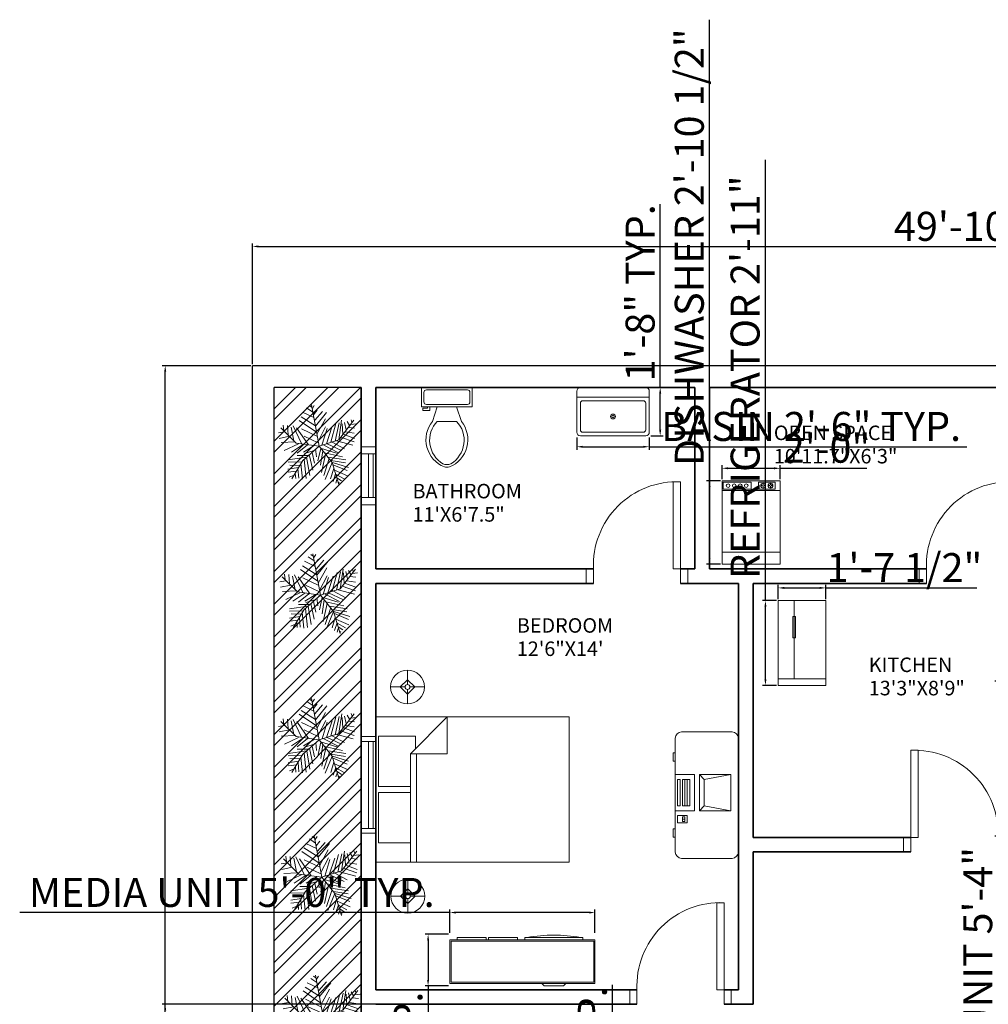
# Model space of a CAD drawing. Units: inches. Extents: x 2297 to 3143, y 440 to 1351.
# Tile 5 of 6: x 2297 to 2697, y 944 to 1351. Entities that reach past the tile are written whole.
import ezdxf

# ---------------------------------------------------------------- set-up
doc = ezdxf.new("R2010")
doc.units = ezdxf.units.IN
for name, color, linetype, lineweight in [('A-ANNO-DIMS', 2, 'Continuous', 18), ('A-AREA-IDEN', 7, 'Continuous', 18), ('A-DOOR', 4, 'Continuous', 20), ('A-EQPM', 8, 'Continuous', 18), ('A-FLOR-FIXT', 9, 'Continuous', 18), ('A-FURN', 8, 'Continuous', 18), ('A-GLAZ', 4, 'Continuous', 18), ('A-WALL', 7, 'Continuous', 35), ('C-PROP', 7, 'Continuous', 25), ('C-SITE-PATT', 252, 'Continuous', 13), ('E-LITE', 9, 'Continuous', 13), ('L-PLNT', 3, 'Continuous', 13)]:
    doc.layers.add(name, color=color, linetype=linetype, lineweight=lineweight)
doc.styles.get("Standard").update_dxf_attribs({"font": 'arial.ttf'})
doc.dimstyles.new('ISO-25', dxfattribs={"dimtxt": 12, "dimasz": 2.5, "dimexe": 1.25, "dimexo": 0.625, "dimtad": 1, "dimdec": 1, "dimlunit": 3, "dimtxsty": 'Standard', "dimcen": 2.5, "dimadec": 0, "dimazin": 0, "dimtfac": 1, "dimtdec": 1, "dimtmove": 0, "dimatfit": 3, "dimfxl": 1, "dimarcsym": 0})

# ---------------------------------------------------------------- blocks, each defined once
blk = doc.blocks.new('Bed - Queen')
for p, q in [((0, -80.00003), (0, 0)), ((0, 0), (59.99999, 0)), ((59.99999, 0), (59.99999, -80.00003)), ((7.99999, -1.2), (28.79998, -1.2)), ((7.99999, -14.4), (7.99999, -1.2)), ((28.79998, -1.2), (28.79998, -14.4)), ((31.19999, -1.2), (51.99999, -1.2)), ((31.19999, -14.4), (31.19999, -1.2)), ((51.99999, -1.2), (51.99999, -16.4)), ((0, -14.4), (44.8, -14.4)), ((59.99999, -29.6), (44.8, -14.4)), ((44.8, -14.4), (44.8, -29.6)), ((44.8, -16.8), (0, -16.8)), ((51.99999, -16.4), (46.79936, -16.4)), ((44.8, -29.6), (59.99999, -29.6)), ((59.99999, -80.00003), (0, -80.00003))]:
    blk.add_line(p, q)
blk = doc.blocks.new('Sink-single - 30 in top')
blk.add_line((-15, -3.999996), (15, -3.999996))
for points in [[(-13.5, 0), (13.5, 0)], [(-15, -18.499996), (-15, -1.5)], [(15, -1.5), (15, -18.499996)], [(-13.5, -17.499996), (-13.5, -6.499996)], [(-12.5, -5.499996), (12.5, -5.499996)], [(13.5, -6.499996), (13.5, -17.499996)], [(13.5, -19.999996), (-13.5, -19.999996)], [(12.5, -18.499996), (-12.5, -18.499996)]]:
    blk.add_lwpolyline(points)
for radius in [1, 0.5]:
    blk.add_circle((0, -11.999996), radius)
for centre, radius, start, end in [((-13.5, -1.5), 1.5, 90, 180), ((13.5, -1.5), 1.5, 0, 90), ((-12.5, -6.499996), 1, 90, 180), ((12.5, -6.499996), 1, 0, 90), ((-13.5, -18.499996), 1.5, 180, 270), ((-12.5, -17.499996), 1, 180, 270), ((12.5, -17.499996), 1, 270, 0), ((13.5, -18.499996), 1.5, 270, 0)]:
    blk.add_arc(centre, radius, start, end)
blk = doc.blocks.new('Toilet - top')
for p, q in [((9.5, -6), (9.5, -2)), ((-8, -8.5), (-8, -8)), ((-7, -8), (-7, -9.5)), ((-4, -8), (-6, -14)), ((4, -8), (6, -14)), ((-10, -8.5), (-8, -8.5)), ((-10, -9.5), (-10, -8.5)), ((-7, -9.5), (-10, -9.5)), ((4, -14), (-4, -14))]:
    blk.add_line(p, q)
blk.add_lwpolyline([(10.5, -8), (10.5, 0), (-10.5, 0), (-10.5, -8)], close=True)
for points in [[(-9.5, -2), (-9.5, -6)], [(8.5, -1), (-8.5, -1)], [(-8.5, -7), (8.5, -7)]]:
    blk.add_lwpolyline(points)
for centre, radius, start, end in [((-8.62, -1.88), 0.884, 81.8699, 188.1301), ((8.62, -1.88), 0.884, 351.8699, 98.1301), ((-8.62, -6.12), 0.884, 171.8699, 278.1301), ((8.62, -6.12), 0.884, 261.8699, 8.1301), ((3.52, -21.58), 12.17, 141.4691, 247.9714), ((4.2, -21.82), 11.33, 136.3677, 238.9468), ((-3.52, -21.58), 12.17, 292.0284, 38.5307), ((-4.2, -21.82), 11.33, 301.053, 43.6321), ((0, -27.88), 4, 245.7318, 294.2682), ((0, -29), 4, 254.8605, 285.1395)]:
    blk.add_arc(centre, radius, start, end)
blk = doc.blocks.new('*U16')
for p, q in [((-10.186, 53.64), (-13.084, 55.962)), ((0, 0), (-10.5, 57)), ((-9.099, 51.782), (-6.563, 55.962)), ((-7.288, 39.707), (-21.778, 46.673)), ((-8.737, 47.138), (-17.069, 52.711)), ((-7.65, 43.423), (-2.578, 49.46)), ((-5.839, 35.992), (4.667, 48.067)), ((-5.114, 27.632), (10.463, 46.673)), ((-48.585, 21.131), (-49.309, 29.026)), ((-43.513, 28.561), (-42.427, 15.558)), ((-35.544, 28.097), (-24.314, 3.947)), ((-3.665, 19.273), (-27.574, 35.527)), ((-5.114, 28.097), (-24.676, 40.636)), ((-2.941, 16.486), (8.652, 37.85)), ((16.259, 5.805), (23.142, 31.348)), ((22.055, 7.198), (27.489, 32.277)), ((27, 9), (48, 36)), ((27.127, 9.056), (31.112, 35.992)), ((31.836, 30.883), (32.561, 16.486)), ((35.096, 32.741), (37.27, 22.524)), ((38.719, 34.134), (41.979, 28.561)), ((43.791, 29.954), (51.036, 30.883)), ((44.153, 36.456), (45.239, 32.741)), ((-47.498, 19.737), (-55.83, 18.344)), ((-40.615, 13.7), (-55.105, 10.913)), ((-31.5, 4.5), (-52.5, 25.5)), ((-38.442, 26.239), (-34.819, 7.663)), ((-14.533, 2.09), (-30.834, 25.31)), ((-24.314, 23.917), (-2.941, 13.7)), ((-20.691, 13.7), (-1.129, 4.876)), ((-1.129, 6.734), (9.014, 26.704)), ((3.942, 1.625), (11.187, 24.381)), ((10.101, 3.483), (17.708, 26.239)), ((33.285, 16.486), (48.862, 10.913)), ((36.183, 19.737), (48.137, 17.88)), ((40.53, 25.775), (48.862, 24.846)), ((-33.37, 6.269), (-52.207, 5.34)), ((-28.299, 3.483), (-47.86, -5.805)), ((-21.416, 3.018), (-38.079, -8.128)), ((0, 0), (-31.5, 4.5)), ((-15.982, 2.09), (-30.11, -9.521)), ((0, 0), (-22.5, -19.5)), ((-6.563, 1.161), (-21.416, -8.128)), ((0, 0), (27, 9)), ((0, 0), (18, -22.5)), ((6.478, 1.625), (26.04, -8.592)), ((11.187, 3.483), (30.749, -5.805)), ((18.07, 5.805), (35.096, -3.483)), ((24.229, 7.663), (46.688, 1.625)), ((29.662, 12.307), (48.137, 6.269)), ((-15.257, -12.772), (-30.11, -12.772)), ((-6.563, -5.805), (-19.967, -9.985)), ((-13.446, -11.378), (-8.737, -32.741)), ((-9.461, -8.592), (-6.201, -23.453)), ((-4.752, -3.483), (-3.665, -14.629)), ((2.493, -3.019), (-1.491, -20.202)), ((1.769, -2.555), (24.229, -9.521)), ((5.029, -6.27), (2.131, -25.775)), ((9.014, -11.378), (3.58, -35.992)), ((7.565, -9.056), (32.198, -14.629)), ((-17.431, -15.094), (-42.789, -18.809)), ((-24.314, -21.596), (-42.427, -22.06)), ((-26.849, -26.24), (-40.253, -25.775)), ((-22.5, -19.5), (-37.5, -45)), ((-25.038, -23.918), (-22.865, -45.281)), ((-20.691, -18.345), (-17.793, -44.352)), ((-17.069, -15.094), (-12.721, -40.172)), ((14.085, -16.951), (6.478, -40.172)), ((18.07, -22.524), (8.289, -45.745)), ((12.274, -15.094), (36.907, -18.809)), ((16.259, -19.738), (36.183, -22.989)), ((18, -22.5), (27, -52.5)), ((18.433, -22.524), (40.53, -29.026)), ((19.157, -25.311), (38.719, -33.206)), ((-28.299, -29.026), (-42.789, -31.348)), ((-30.834, -34.135), (-42.427, -35.528)), ((-34.457, -39.708), (-40.978, -42.494)), ((-32.646, -36.921), (-31.921, -44.352)), ((-29.023, -30.884), (-27.936, -43.887)), ((20.244, -30.419), (15.897, -44.816)), ((22.78, -37.85), (19.519, -48.532)), ((21.331, -32.741), (39.081, -40.636)), ((22.78, -38.314), (34.372, -44.816)), ((24.591, -45.745), (23.142, -50.854)), ((24.591, -43.423), (30.749, -47.603)), ((26.764, -49.925), (28.213, -50.854))]:
    blk.add_line(p, q)
blk = doc.blocks.new('*D17')
at = {"layer": 'A-ANNO-DIMS', "color": 0, "lineweight": -2, "transparency": 16777216}
for p, q in [((2393.19, 1208.26), (2393.19, 1258.2)), ((2991.69, 1208.26), (2991.69, 1258.2)), ((2395.69, 1256.95), (2989.19, 1256.95))]:
    blk.add_line(p, q, dxfattribs=at)
at = {"layer": 'A-ANNO-DIMS', "color": 0, "transparency": 16777216}
for points in [[(2395.69, 1257.36), (2395.69, 1256.53), (2393.19, 1256.95)], [(2989.19, 1257.36), (2989.19, 1256.53), (2991.69, 1256.95)]]:
    blk.add_solid(points, dxfattribs=at)
at = {"layer": 'Defpoints', "color": 0, "transparency": 16777216}
for p in [(2991.69, 1256.95), (2393.19, 1207.63), (2991.69, 1207.63)]:
    blk.add_point(p, dxfattribs=at)
at = {"layer": 'A-ANNO-DIMS', "color": 0, "transparency": 16777216, "insert": (2692.44, 1263.7), "char_height": 12, "attachment_point": 5}
blk.add_mtext('49\'-10.5"', dxfattribs=at)
blk = doc.blocks.new('Lamp - Table')
for p, q in [((0, 7), (0, 1)), ((-1, 0), (-7, 0)), ((0, 3), (-3, 0)), ((-3, 0), (0, -3)), ((3, 0), (0, 3)), ((0, -3), (3, 0)), ((1, 0), (7, 0)), ((0, -1), (0, -7))]:
    blk.add_line(p, q)
for radius in [7, 1]:
    blk.add_circle((0, 0), radius)
blk = doc.blocks.new('Refrigerator-2 door - 36 in front')
for p, q in [((12, 5), (12, 64)), ((0, 5), (36, 5))]:
    blk.add_line(p, q)
for points in [[(0, 0), (0, 64), (36, 64), (36, 0)], [(11, 36), (11, 52), (13, 52), (13, 36)]]:
    blk.add_lwpolyline(points, close=True)
blk = doc.blocks.new('Desk - 30 x 60 in.')
for p, q in [((-26.999995, 0), (26.999995, 0)), ((-29.999995, -27), (-29.999995, -3)), ((29.999995, -3), (29.999995, -27)), ((26.999995, -30), (-26.999995, -30)), ((-20.000005, -30), (-20.000005, -31)), ((-20.000005, -31), (-16.000005, -31)), ((-16.000005, -31), (-16.000005, -30)), ((15.999995, -31), (15.999995, -30)), ((19.999995, -31), (15.999995, -31)), ((19.999995, -30), (19.999995, -31))]:
    blk.add_line(p, q)
for centre, start, end in [((-26.499995, -3.5), 98.1301, 171.8699), ((26.499995, -3.5), 8.130102, 81.8699), ((-26.499995, -26.5), 188.1301, 261.8699), ((26.499995, -26.5), 278.1301, 351.8699)]:
    blk.add_arc(centre, 3.535534, start, end)
blk = doc.blocks.new('Computer Terminal')
for p, q in [((-10, 11.5), (5, 11.5)), ((-8, 0.5), (-10, 11.5)), ((-10, -1.5), (-10, 11.5)), ((5, 11.5), (3, 0.5)), ((5, 11.5), (5, -1.5)), ((-10, -1.5), (-8, 0.5)), ((3, 0.5), (-8, 0.5)), ((3, 0.5), (5, -1.5)), ((5, -1.5), (-10, -1.5)), ((-10, -11.5), (-10, -3.5)), ((-10, -3.5), (5, -3.5)), ((5, -3.5), (5, -11.5)), ((-8, -5.5), (-8, -8.5)), ((3, -5.5), (-8, -5.5)), ((3, -6.5), (-8, -6.5)), ((-8, -7.5), (3, -7.5)), ((3, -8.5), (3, -5.5)), ((10, -6.5), (7, -6.5)), ((7, -6.5), (7, -10.5)), ((9.5, -7.5), (7.5, -7.5)), ((7.5, -7.5), (7.5, -8.5)), ((8.5, -7.5), (8.5, -8.5)), ((9.5, -8.5), (9.5, -7.5)), ((10, -10.5), (10, -6.5)), ((5, -11.5), (-10, -11.5)), ((-8, -8.5), (3, -8.5)), ((-8, -9.5), (-8, -10.5)), ((3, -9.5), (-8, -9.5)), ((-8, -10.5), (3, -10.5)), ((3, -10.5), (3, -9.5)), ((7, -10.5), (10, -10.5)), ((7.5, -8.5), (9.5, -8.5))]:
    blk.add_line(p, q)
blk = doc.blocks.new('Dishwasher')
for p, q in [((16.3156, 33.1843), (16.5, 33)), ((17, 32.75), (17, 33.5)), ((17.5, 33), (17.6938, 33.1938)), ((19.3156, 33.1843), (19.5, 33)), ((20, 32.75), (20, 33.5)), ((20.5, 33), (20.6938, 33.1938)), ((24, 30.5), (0, 30.5)), ((16, 32.5), (16.75, 32.5)), ((16.5, 32), (16.2942, 31.7942)), ((17, 32.25), (17, 31.5)), ((18, 32.5), (17.25, 32.5)), ((17.7061, 31.7939), (17.5, 32)), ((19, 32.5), (19.75, 32.5)), ((19.5, 32), (19.2942, 31.7942)), ((20, 32.25), (20, 31.5)), ((21, 32.5), (20.25, 32.5)), ((20.7061, 31.7939), (20.5, 32)), ((0, 5), (24, 5))]:
    blk.add_line(p, q)
for points in [[(0, 0), (0, 34.5), (24, 34.5), (24, 0)], [(0.5, 31), (0.5, 34), (12, 34), (12, 31)], [(15, 31), (15, 34), (22, 34), (22, 31)]]:
    blk.add_lwpolyline(points, close=True)
for centre, radius in [((2.5, 32.5), 0.75), ((5, 32.5), 0.75), ((7.5, 32.5), 0.75), ((10, 32.5), 0.75), ((17, 32.5), 1), ((20, 32.5), 1)]:
    blk.add_circle(centre, radius)
blk = doc.blocks.new('Entertainment Center')
for p, q in [((-4, 0), (-5, -1)), ((4, 0), (-4, 0)), ((5, -1), (4, 0)), ((-17, -19), (-17, -1)), ((-17, -1), (43, -1)), ((-16.5, -18.5), (-16.5, -1.5)), ((-16.5, -1.5), (42.5, -1.5)), ((42.5, -1.5), (42.5, -18.5)), ((43, -1), (43, -19)), ((43, -19), (-17, -19)), ((42.5, -18.5), (-16.5, -18.5)), ((-12, -20), (-12, -19)), ((12, -20), (-12, -20)), ((12, -19), (12, -20)), ((15, -20), (15, -19)), ((27, -20), (15, -20)), ((27, -19), (27, -20)), ((28, -20), (28, -19)), ((40, -20), (28, -20)), ((40, -19), (40, -20))]:
    blk.add_line(p, q)
blk.add_arc((0, 40), 61, 259.6111, 280.3889)
blk = doc.blocks.new('DOOR-36IN-6IN-JAMB')
for p, q in [((0, 6), (0, 0)), ((3, 6), (3, 0)), ((39, 6), (39, 0)), ((42, 6), (42, 0))]:
    blk.add_line(p, q)
blk.add_lwpolyline([(39, 6), (36, 6), (36, 42), (39, 42)], close=True)
blk.add_arc((37.5, 7.5), 34.53, 87.5104, 182.4896)
blk = doc.blocks.new('WIN-36IN-6IN-WALL')
for p, q in [((6, 40), (0, 40)), ((6, 38), (0, 38)), ((3, 38), (3, 2)), ((5, 38), (5, 2)), ((0, 2), (6, 2)), ((0, 0), (6, 0))]:
    blk.add_line(p, q)
blk = doc.blocks.new('WIN-18IN-6IN-WALL')
for p, q in [((6, 24), (0, 24)), ((6, 21), (0, 21)), ((1, 3), (1, 21)), ((3, 3), (3, 21)), ((0, 3), (6, 3)), ((0, 0), (6, 0))]:
    blk.add_line(p, q)
blk = doc.blocks.new('*D34')
at = {"layer": 'A-ANNO-DIMS', "color": 0, "lineweight": -2, "transparency": 16777216}
for p, q in [((2542.03, 874.63), (2542.03, 951.74)), ((2534.79, 874.63), (2543.28, 874.63)), ((2542.03, 850.07), (2542.03, 872.13)), ((2534.79, 847.57), (2543.28, 847.57))]:
    blk.add_line(p, q, dxfattribs=at)
at = {"layer": 'A-ANNO-DIMS', "color": 0, "transparency": 16777216}
for points in [[(2541.61, 872.13), (2542.44, 872.13), (2542.03, 874.63)], [(2541.61, 850.07), (2542.44, 850.07), (2542.03, 847.57)]]:
    blk.add_solid(points, dxfattribs=at)
at = {"layer": 'Defpoints', "color": 0, "transparency": 16777216}
for p in [(2534.17, 874.63), (2542.03, 874.63), (2534.17, 847.57)]:
    blk.add_point(p, dxfattribs=at)
at = {"layer": 'A-ANNO-DIMS', "color": 0, "transparency": 16777216, "insert": (2535.27, 914.43), "char_height": 12, "attachment_point": 5, "rotation": 90}
blk.add_mtext('2\'-3" TYP.', dxfattribs=at)
blk = doc.blocks.new('*D39')
at = {"layer": 'A-ANNO-DIMS', "color": 0, "lineweight": -2, "transparency": 16777216}
for p, q in [((2527.3, 1178.01), (2527.3, 1172.88)), ((2557.3, 1178.01), (2557.3, 1172.88)), ((2529.8, 1174.13), (2554.8, 1174.13)), ((2557.3, 1174.13), (2688.63, 1174.13))]:
    blk.add_line(p, q, dxfattribs=at)
at = {"layer": 'A-ANNO-DIMS', "color": 0, "transparency": 16777216}
for points in [[(2529.8, 1174.55), (2529.8, 1173.72), (2527.3, 1174.13)], [(2554.8, 1174.55), (2554.8, 1173.72), (2557.3, 1174.13)]]:
    blk.add_solid(points, dxfattribs=at)
at = {"layer": 'Defpoints', "color": 0, "transparency": 16777216}
for p in [(2527.3, 1178.63), (2557.3, 1178.63), (2557.3, 1174.13)]:
    blk.add_point(p, dxfattribs=at)
at = {"layer": 'A-ANNO-DIMS', "color": 0, "transparency": 16777216, "insert": (2624.22, 1180.96), "char_height": 12, "attachment_point": 5}
blk.add_mtext('BASIN 2\'-6" TYP.', dxfattribs=at)
blk = doc.blocks.new('*D40')
at = {"layer": 'A-ANNO-DIMS', "color": 0, "lineweight": -2, "transparency": 16777216}
for p, q in [((2561.8, 1198.63), (2561.8, 1274.4)), ((2557.93, 1198.63), (2563.05, 1198.63)), ((2561.8, 1181.13), (2561.8, 1196.13)), ((2557.93, 1178.63), (2563.05, 1178.63))]:
    blk.add_line(p, q, dxfattribs=at)
at = {"layer": 'A-ANNO-DIMS', "color": 0, "transparency": 16777216}
for points in [[(2561.39, 1196.13), (2562.22, 1196.13), (2561.8, 1198.63)], [(2561.39, 1181.13), (2562.22, 1181.13), (2561.8, 1178.63)]]:
    blk.add_solid(points, dxfattribs=at)
at = {"layer": 'Defpoints', "color": 0, "transparency": 16777216}
for p in [(2557.3, 1198.63), (2561.8, 1198.63), (2557.3, 1178.63)]:
    blk.add_point(p, dxfattribs=at)
at = {"layer": 'A-ANNO-DIMS', "color": 0, "transparency": 16777216, "insert": (2555.05, 1237.77), "char_height": 12, "attachment_point": 5, "rotation": 90}
blk.add_mtext('1\'-8" TYP.', dxfattribs=at)
blk = doc.blocks.new('*D41')
at = {"layer": 'A-ANNO-DIMS', "color": 0, "lineweight": -2, "transparency": 16777216}
for p, q in [((2474.84, 981.57), (2296.97, 981.57)), ((2474.84, 973.2), (2474.84, 982.82)), ((2532.34, 981.57), (2477.34, 981.57)), ((2534.84, 973.2), (2534.84, 982.82))]:
    blk.add_line(p, q, dxfattribs=at)
at = {"layer": 'A-ANNO-DIMS', "color": 0, "transparency": 16777216}
for points in [[(2477.34, 981.99), (2477.34, 981.16), (2474.84, 981.57)], [(2532.34, 981.99), (2532.34, 981.16), (2534.84, 981.57)]]:
    blk.add_solid(points, dxfattribs=at)
at = {"layer": 'Defpoints', "color": 0, "transparency": 16777216}
for p in [(2474.84, 981.57), (2474.84, 972.57), (2534.84, 972.57)]:
    blk.add_point(p, dxfattribs=at)
at = {"layer": 'A-ANNO-DIMS', "color": 0, "transparency": 16777216, "insert": (2384.65, 988.33), "char_height": 12, "attachment_point": 5}
blk.add_mtext('MEDIA UNIT 5\'-0" TYP.', dxfattribs=at)
blk = doc.blocks.new('*D42')
at = {"layer": 'A-ANNO-DIMS', "color": 0, "lineweight": -2, "transparency": 16777216}
for p, q in [((2474.21, 972.57), (2464.59, 972.57)), ((2465.84, 970.07), (2465.84, 953.74)), ((2474.21, 951.24), (2464.59, 951.24)), ((2465.84, 951.24), (2465.84, 847.51))]:
    blk.add_line(p, q, dxfattribs=at)
at = {"layer": 'A-ANNO-DIMS', "color": 0, "transparency": 16777216}
for points in [[(2465.42, 970.07), (2466.25, 970.07), (2465.84, 972.57)], [(2465.42, 953.74), (2466.25, 953.74), (2465.84, 951.24)]]:
    blk.add_solid(points, dxfattribs=at)
at = {"layer": 'Defpoints', "color": 0, "transparency": 16777216}
for p in [(2474.84, 972.57), (2465.84, 951.24), (2474.84, 951.24)]:
    blk.add_point(p, dxfattribs=at)
at = {"layer": 'A-ANNO-DIMS', "color": 0, "transparency": 16777216, "insert": (2459.01, 898.13), "char_height": 12, "attachment_point": 5, "rotation": 90}
blk.add_mtext('1\'-9 1/2" TYP.', dxfattribs=at)
blk = doc.blocks.new('*D61')
at = {"layer": 'A-ANNO-DIMS', "color": 0, "lineweight": -2, "transparency": 16777216}
for p, q in [((2710.47, 1077.25), (2700.22, 1077.25)), ((2701.47, 1074.75), (2701.47, 1015.6)), ((2710.47, 1013.1), (2700.22, 1013.1)), ((2701.47, 1013.1), (2701.47, 855.98))]:
    blk.add_line(p, q, dxfattribs=at)
at = {"layer": 'A-ANNO-DIMS', "color": 0, "transparency": 16777216}
for points in [[(2701.05, 1074.75), (2701.89, 1074.75), (2701.47, 1077.25)], [(2701.05, 1015.6), (2701.89, 1015.6), (2701.47, 1013.1)]]:
    blk.add_solid(points, dxfattribs=at)
at = {"layer": 'Defpoints', "color": 0, "transparency": 16777216}
for p in [(2711.09, 1077.25), (2701.47, 1013.1), (2711.09, 1013.1)]:
    blk.add_point(p, dxfattribs=at)
at = {"layer": 'A-ANNO-DIMS', "color": 0, "transparency": 16777216, "insert": (2694.64, 933.29), "char_height": 12, "attachment_point": 5, "rotation": 90}
blk.add_mtext('KITCHEN UNIT 5\'-4"', dxfattribs=at)
blk = doc.blocks.new('*D65')
at = {"layer": 'A-ANNO-DIMS', "color": 0, "lineweight": -2, "transparency": 16777216}
for p, q in [((2605.32, 1110.52), (2605.32, 1292.72)), ((2609.94, 1110.52), (2604.07, 1110.52)), ((2605.32, 1077.99), (2605.32, 1108.02)), ((2609.94, 1075.49), (2604.07, 1075.49))]:
    blk.add_line(p, q, dxfattribs=at)
at = {"layer": 'A-ANNO-DIMS', "color": 0, "transparency": 16777216}
for points in [[(2604.9, 1108.02), (2605.73, 1108.02), (2605.32, 1110.52)], [(2604.9, 1077.99), (2605.73, 1077.99), (2605.32, 1075.49)]]:
    blk.add_solid(points, dxfattribs=at)
at = {"layer": 'Defpoints', "color": 0, "transparency": 16777216}
for p in [(2605.32, 1110.52), (2610.57, 1110.52), (2610.57, 1075.49)]:
    blk.add_point(p, dxfattribs=at)
at = {"layer": 'A-ANNO-DIMS', "color": 0, "transparency": 16777216, "insert": (2598.48, 1202.87), "char_height": 12, "attachment_point": 5, "rotation": 90}
blk.add_mtext('REFRIGERATOR 2\'-11"', dxfattribs=at)
blk = doc.blocks.new('*D66')
at = {"layer": 'A-ANNO-DIMS', "color": 0, "lineweight": -2, "transparency": 16777216}
for p, q in [((2610.57, 1111.15), (2610.57, 1117.03)), ((2613.07, 1115.78), (2627.78, 1115.78)), ((2630.28, 1111.15), (2630.28, 1117.03)), ((2630.28, 1115.78), (2692.76, 1115.78))]:
    blk.add_line(p, q, dxfattribs=at)
at = {"layer": 'A-ANNO-DIMS', "color": 0, "transparency": 16777216}
for points in [[(2613.07, 1116.2), (2613.07, 1115.36), (2610.57, 1115.78)], [(2627.78, 1116.2), (2627.78, 1115.36), (2630.28, 1115.78)]]:
    blk.add_solid(points, dxfattribs=at)
at = {"layer": 'Defpoints', "color": 0, "transparency": 16777216}
for p in [(2630.28, 1115.78), (2610.57, 1110.52), (2630.28, 1110.52)]:
    blk.add_point(p, dxfattribs=at)
at = {"layer": 'A-ANNO-DIMS', "color": 0, "transparency": 16777216, "insert": (2662.77, 1122.61), "char_height": 12, "attachment_point": 5}
blk.add_mtext('1\'-7 1/2"', dxfattribs=at)
blk = doc.blocks.new('*D67')
at = {"layer": 'A-ANNO-DIMS', "color": 0, "lineweight": -2, "transparency": 16777216}
for p, q in [((2582.21, 1160.06), (2582.21, 1350.68)), ((2586.76, 1160.06), (2580.96, 1160.06)), ((2582.21, 1128.06), (2582.21, 1157.56)), ((2586.76, 1125.56), (2580.96, 1125.56))]:
    blk.add_line(p, q, dxfattribs=at)
at = {"layer": 'A-ANNO-DIMS', "color": 0, "transparency": 16777216}
for points in [[(2581.8, 1157.56), (2582.63, 1157.56), (2582.21, 1160.06)], [(2581.8, 1128.06), (2582.63, 1128.06), (2582.21, 1125.56)]]:
    blk.add_solid(points, dxfattribs=at)
at = {"layer": 'Defpoints', "color": 0, "transparency": 16777216}
for p in [(2582.21, 1160.06), (2587.39, 1160.06), (2587.39, 1125.56)]:
    blk.add_point(p, dxfattribs=at)
at = {"layer": 'A-ANNO-DIMS', "color": 0, "transparency": 16777216, "insert": (2575.39, 1256.62), "char_height": 12, "attachment_point": 5, "rotation": 90}
blk.add_mtext('DISHWASHER 2\'-10 1/2"', dxfattribs=at)
blk = doc.blocks.new('*D68')
at = {"layer": 'A-ANNO-DIMS', "color": 0, "lineweight": -2, "transparency": 16777216}
for p, q in [((2587.39, 1160.68), (2587.39, 1166.48)), ((2589.89, 1165.23), (2608.89, 1165.23)), ((2611.39, 1160.68), (2611.39, 1166.48)), ((2611.39, 1165.23), (2647.24, 1165.23))]:
    blk.add_line(p, q, dxfattribs=at)
at = {"layer": 'A-ANNO-DIMS', "color": 0, "transparency": 16777216}
for points in [[(2589.89, 1165.65), (2589.89, 1164.81), (2587.39, 1165.23)], [(2608.89, 1165.65), (2608.89, 1164.81), (2611.39, 1165.23)]]:
    blk.add_solid(points, dxfattribs=at)
at = {"layer": 'Defpoints', "color": 0, "transparency": 16777216}
for p in [(2611.39, 1165.23), (2587.39, 1160.06), (2611.39, 1160.06)]:
    blk.add_point(p, dxfattribs=at)
at = {"layer": 'A-ANNO-DIMS', "color": 0, "transparency": 16777216, "insert": (2630.57, 1171.98), "char_height": 12, "attachment_point": 5}
blk.add_mtext('2\'-0"', dxfattribs=at)
blk = doc.blocks.new('*D70')
at = {"layer": 'A-ANNO-DIMS', "color": 0, "lineweight": -2, "transparency": 16777216}
for p, q in [((2392.57, 1207.63), (2355.89, 1207.63)), ((2357.14, 583.13), (2357.14, 1205.13)), ((2437.57, 580.63), (2355.89, 580.63))]:
    blk.add_line(p, q, dxfattribs=at)
at = {"layer": 'A-ANNO-DIMS', "color": 0, "transparency": 16777216}
for points in [[(2356.73, 1205.13), (2357.56, 1205.13), (2357.14, 1207.63)], [(2356.73, 583.13), (2357.56, 583.13), (2357.14, 580.63)]]:
    blk.add_solid(points, dxfattribs=at)
at = {"layer": 'Defpoints', "color": 0, "transparency": 16777216}
for p in [(2357.14, 1207.63), (2393.19, 1207.63), (2438.19, 580.63)]:
    blk.add_point(p, dxfattribs=at)
at = {"layer": 'A-ANNO-DIMS', "color": 0, "transparency": 16777216, "insert": (2350.39, 894.13), "char_height": 12, "attachment_point": 5, "rotation": 90}
blk.add_mtext('52\'-3"', dxfattribs=at)
blk = doc.blocks.new('*D78')
at = {"layer": 'A-ANNO-DIMS', "color": 0, "lineweight": -2, "transparency": 16777216}
for p, q in [((2548.57, 943.63), (2355.89, 943.63)), ((2357.14, 883.13), (2357.14, 941.13)), ((2548.57, 880.63), (2355.89, 880.63))]:
    blk.add_line(p, q, dxfattribs=at)
at = {"layer": 'A-ANNO-DIMS', "color": 0, "transparency": 16777216}
for points in [[(2356.73, 941.13), (2357.56, 941.13), (2357.14, 943.63)], [(2356.73, 883.13), (2357.56, 883.13), (2357.14, 880.63)]]:
    blk.add_solid(points, dxfattribs=at)
at = {"layer": 'Defpoints', "color": 0, "transparency": 16777216}
for p in [(2357.14, 943.63), (2549.19, 943.63), (2549.19, 880.63)]:
    blk.add_point(p, dxfattribs=at)
at = {"layer": 'A-ANNO-DIMS', "color": 0, "transparency": 16777216, "insert": (2350.39, 912.13), "char_height": 12, "attachment_point": 5, "rotation": 90}
blk.add_mtext('5\'-3"', dxfattribs=at)

msp = doc.modelspace()

# ---------------------------------------------------------------- hatches: boundary and pattern name
at = {"layer": 'C-SITE-PATT'}
h = msp.add_hatch(dxfattribs=at)
h.set_pattern_fill('ANSI32', color=256)
h.paths.add_polyline_path([(2438.19, 1198.63), (2402.19, 1198.63), (2402.19, 556.63), (2667.43, 556.63), (2742.43, 556.63), (2946.69, 556.63), (2982.69, 556.63), (2982.69, 1117.63), (2982.69, 1123.63), (2982.69, 1198.63), (2946.69, 1198.63), (2946.69, 1117.63), (2946.69, 700.63), (2806.19, 700.63), (2806.19, 580.63), (2738.57, 580.63), (2738.57, 589.63), (2735.57, 589.63), (2735.57, 625.63, 0.402069), (2702.6, 591.13, 0.401544), (2669.57, 625.63), (2669.57, 589.63), (2666.57, 589.63), (2666.57, 580.63), (2438.19, 580.63)])
h.paths.add_polyline_path([(2706.46, 558.2, -0.000472), (2706.46, 558.13, -0.000473)], flags=16)
h.paths.add_polyline_path([(2875.15, 576.11), (2920.92, 576.11), (2920.92, 585.31), (2875.15, 585.31)], flags=24)
h.paths.add_polyline_path([(2875.13, 585.74), (2915.96, 585.74), (2915.96, 595.05), (2875.13, 595.05)], flags=24)
h.paths.add_polyline_path([(2646.52, 1069.72), (2687.63, 1069.72), (2687.63, 1078.92), (2646.52, 1078.92)], flags=25)
h.paths.add_polyline_path([(2646.5, 1079.35), (2686.39, 1079.35), (2686.39, 1088.65), (2646.5, 1088.65)], flags=25)

# ---------------------------------------------------------------- linework, layer by layer
at = {"layer": 'A-WALL'}
for p, q in [((2438.19, 580.63), (2438.19, 1198.63)), ((2576.19, 1198.63), (2444.19, 1198.63)), ((2444.19, 1123.63), (2444.19, 1198.63)), ((2576.19, 1123.63), (2576.19, 1198.63)), ((2582.19, 1123.63), (2582.19, 1198.63)), ((2713.89, 1198.63), (2582.19, 1198.63)), ((2534.19, 1123.63), (2444.19, 1123.63)), ((2576.19, 1123.63), (2570.19, 1123.63)), ((2671.89, 1123.63), (2582.19, 1123.63)), ((2444.19, 949.63), (2444.19, 1117.63)), ((2534.19, 1117.63), (2444.19, 1117.63)), ((2594.19, 1117.63), (2570.19, 1117.63)), ((2594.19, 949.63), (2594.19, 1117.63)), ((2600.19, 1012.63), (2600.19, 1117.63)), ((2671.89, 1117.63), (2600.19, 1117.63)), ((2665.46, 1012.63), (2600.19, 1012.63)), ((2600.19, 943.63), (2600.19, 1006.63)), ((2665.46, 1006.63), (2600.19, 1006.63)), ((2552.19, 949.63), (2444.19, 949.63)), ((2594.19, 949.63), (2588.19, 949.63)), ((2552.19, 943.63), (2444.19, 943.63)), ((2600.19, 943.63), (2588.19, 943.63))]:
    msp.add_line(p, q, dxfattribs=at)
at = {"layer": 'C-PROP'}
for p, q in [((2393.19, 547.63), (2393.19, 1207.63)), ((2402.19, 556.63), (2402.19, 1198.63)), ((2438.19, 1198.63), (2402.19, 1198.63))]:
    msp.add_line(p, q, dxfattribs=at)
msp.add_lwpolyline([(2742.43, 547.63), (2991.69, 547.63), (2991.69, 1207.63), (2393.19, 1207.63)], dxfattribs=at)

# ---------------------------------------------------------------- block references
at = {"layer": 'A-DOOR'}
for p in [(2531.19, 1117.63), (2668.89, 1117.63), (2549.19, 943.63)]:
    msp.add_blockref('DOOR-36IN-6IN-JAMB', p, dxfattribs=at)
at = {"layer": 'A-DOOR', "extrusion": (0, 0, -1), "zscale": -1}
msp.add_blockref('DOOR-36IN-6IN-JAMB', (-2704.46, 1006.63), dxfattribs=at)
at = {"layer": 'A-EQPM'}
msp.add_blockref('Dishwasher', (2587.39, 1125.56), dxfattribs=at)
at = {"layer": 'A-EQPM', "xscale": 0.5473847976192019, "yscale": 0.5473847976192019, "zscale": 0.5473847976192019}
msp.add_blockref('Refrigerator-2 door - 36 in front', (2610.57, 1075.49), dxfattribs=at)
at = {"layer": 'A-EQPM', "rotation": 270}
msp.add_blockref('Computer Terminal', (2579.5, 1028.64), dxfattribs=at)
at = {"layer": 'A-FLOR-FIXT'}
for name, p in [('Toilet - top', (2473.61, 1198.63)), ('Sink-single - 30 in top', (2542.3, 1198.63))]:
    msp.add_blockref(name, p, dxfattribs=at)
at = {"layer": 'A-FURN'}
for name, p, rotation in [('Bed - Queen', (2444.19, 1002.43), 90), ('Entertainment Center', (2517.84, 951.24), 180)]:
    msp.add_blockref(name, p, dxfattribs=dict(at, rotation=rotation))
at = {"layer": 'A-FURN', "xscale": 0.8729228900222988, "yscale": 0.8729228900222988, "zscale": 0.8729228900222988, "rotation": 270}
msp.add_blockref('Desk - 30 x 60 in.', (2594.19, 1030.13), dxfattribs=at)
at = {"layer": 'A-GLAZ', "rotation": 180}
msp.add_blockref('WIN-18IN-6IN-WALL', (2444.19, 1174.16), dxfattribs=at)
at = {"layer": 'A-GLAZ'}
msp.add_blockref('WIN-36IN-6IN-WALL', (2438.19, 1014.32), dxfattribs=at)
at = {"layer": 'E-LITE'}
for p in [(2457.32, 1074.82), (2457.44, 988.34)]:
    msp.add_blockref('Lamp - Table', p, dxfattribs=at)
at = {"layer": 'L-PLNT', "xscale": 0.3005060358918508, "yscale": 0.3005060358918508, "zscale": 0.3005060358918508}
for p in [(2420.75, 1174.33), (2421.33, 1112.74), (2420.79, 1052.94), (2421.89, 996.15), (2422.43, 938.51)]:
    msp.add_blockref('*U16', p, dxfattribs=at)

# ---------------------------------------------------------------- texts
at = {"layer": 'A-AREA-IDEN'}
for s, p in [('OPEN SPACE', (2608.79, 1176.88)), ('10\'11.7"X6\'3"', (2608.79, 1167.24)), ('BATHROOM', (2459.39, 1152.8)), ('11\'X6\'7.5"', (2459.39, 1143.16)), ('BEDROOM', (2502.53, 1097.26)), ('12\'6"X14\'', (2502.53, 1087.63)), ('KITCHEN', (2648.05, 1081)), ('13\'3"X8\'9"', (2648.05, 1071.36))]:
    msp.add_text(s, height=6, dxfattribs=at).set_placement(p)

# ---------------------------------------------------------------- dimensions: what is measured, and where the dimension line sits
at = {"layer": 'A-ANNO-DIMS'}
for base, p1, p2, angle, text, picture, middle in [((2582.21, 1160.06), (2587.39, 1125.56), (2587.39, 1160.06), 90, 'DISHWASHER <>', '*D67', (2575.39, 1256.62)), ((2605.32, 1110.52), (2610.57, 1075.49), (2610.57, 1110.52), 90, 'REFRIGERATOR <>', '*D65', (2598.48, 1202.87)), ((2561.8, 1198.63), (2557.3, 1178.63), (2557.3, 1198.63), 90, '<> TYP.', '*D40', (2555.05, 1237.77)), ((2701.4701, 1013.0979), (2711.0925, 1077.2469), (2711.0925, 1013.0979), 270, 'KITCHEN UNIT <>', '*D61', (2694.6405, 933.2867)), ((2474.84, 981.57), (2534.84, 972.57), (2474.84, 972.57), 180, 'MEDIA UNIT <> TYP.', '*D41', (2384.65, 988.33)), ((2465.84, 951.24), (2474.84, 972.57), (2474.84, 951.24), 270, '<> TYP.', '*D42', (2459.01, 898.13)), ((2542.03, 874.63), (2534.17, 847.57), (2534.17, 874.63), 90, '<> TYP.', '*D34', (2535.27, 914.43))]:
    dim = msp.add_linear_dim(base=base, p1=p1, p2=p2, angle=angle, text=text, dimstyle='ISO-25', override={"dimdec": 1, "dimlfac": 1, "dimrnd": 0, "dimzin": 1, "dimdsep": 46, "dimlunit": 4, "dimfrac": 2}, dxfattribs=at)
    dim.commit()
    dim.dimension.update_dxf_attribs({"geometry": picture, "text_midpoint": middle})
for base, p1, p2, override, picture, middle in [((2991.69, 1256.95), (2393.19, 1207.63), (2991.69, 1207.63), {"dimclrd": 0, "dimclre": 0, "dimclrt": 0}, '*D17', (2692.44, 1263.7)), ((2611.39, 1165.23), (2587.39, 1160.06), (2611.39, 1160.06), {"dimdec": 1, "dimlfac": 1, "dimrnd": 0, "dimzin": 1, "dimdsep": 46, "dimlunit": 4, "dimfrac": 2}, '*D68', (2630.57, 1171.98)), ((2630.28, 1115.78), (2610.57, 1110.52), (2630.28, 1110.52), {"dimdec": 1, "dimlfac": 1, "dimrnd": 0, "dimzin": 1, "dimdsep": 46, "dimlunit": 4, "dimfrac": 2}, '*D66', (2662.77, 1122.61))]:
    dim = msp.add_linear_dim(base=base, p1=p1, p2=p2, dimstyle='ISO-25', override=override, dxfattribs=at)
    dim.commit()
    dim.dimension.update_dxf_attribs({"geometry": picture, "text_midpoint": middle})
for base, p1, p2, picture, middle in [((2357.14, 1207.63), (2438.19, 580.63), (2393.19, 1207.63), '*D70', (2350.39, 894.13)), ((2357.14, 943.63), (2549.19, 880.63), (2549.19, 943.63), '*D78', (2350.39, 912.13))]:
    dim = msp.add_linear_dim(base=base, p1=p1, p2=p2, angle=90, dimstyle='ISO-25', override={"dimdec": 1, "dimlfac": 1, "dimrnd": 0, "dimzin": 1, "dimdsep": 46, "dimlunit": 4, "dimfrac": 2}, dxfattribs=at)
    dim.commit()
    dim.dimension.update_dxf_attribs({"geometry": picture, "text_midpoint": middle})
dim = msp.add_linear_dim(base=(2557.3, 1174.13), p1=(2527.3, 1178.63), p2=(2557.3, 1178.63), text='BASIN <> TYP.', dimstyle='ISO-25', override={"dimdec": 1, "dimlfac": 1, "dimrnd": 0, "dimzin": 1, "dimdsep": 46, "dimlunit": 4, "dimfrac": 2}, dxfattribs=at)
dim.commit()
dim.dimension.update_dxf_attribs({"geometry": '*D39', "text_midpoint": (2624.22, 1180.96)})

doc.saveas('drawing.dxf')
